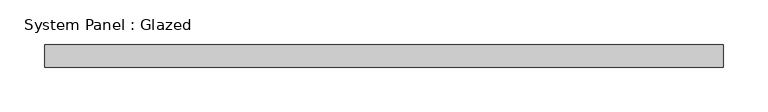
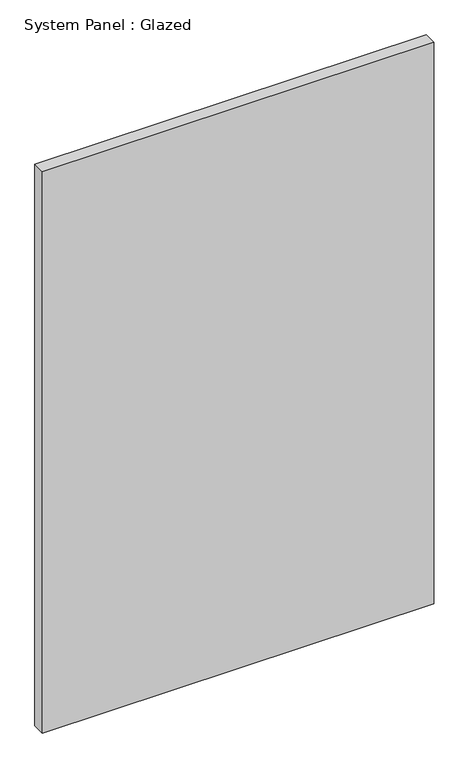
"""IFC4 building model written with IfcOpenShell, lengths in millimetres: plate geometry, System Panel : Glazed."""

from ifc_helpers import new_model, si_unit, origin, origin_with_axes, place, context, project, spatial, polyline, outline, extrude, source, transform, mapped, element, save


def system_panel_glazed_f269d4c8(model_context):
    return source(origin(), model_context, "Body", "SweptSolid", [
        extrude(outline(polyline([(381.0, 19.05), (-381.0, 19.05), (-381.0, 44.45), (381.0, 44.45), (381.0, 19.05)])), origin_with_axes(), (0.0, 0.0, 1.0), 1155.7),
    ])


if __name__ == "__main__":
    model = new_model("IFC4")
    model_context = context("Model", 3, world=origin())
    ifc_project = project(units=[si_unit("LENGTHUNIT", "METRE", prefix="MILLI")], contexts=[model_context])
    site = spatial("IfcSite", under=ifc_project)
    building = spatial("IfcBuilding", under=site)
    placement = place(None, origin())
    system_panel_glazed_shape = system_panel_glazed_f269d4c8(model_context)
    element("IfcPlate", 1, ObjectType="System Panel : Glazed", at=placement, inside=building, context=model_context, shape_type="MappedRepresentation", body=[
        mapped(system_panel_glazed_shape, transform((0.0, 0.0, 0.0), x_axis=(1.0, 0.0, 0.0), y_axis=(0.0, 1.0, 0.0), z_axis=(0.0, 0.0, 1.0))),
    ])
    save(model, "model.ifc")

# Revit data of these elements
# Type "System Panel : Glazed"
#   Construction Type Id = "GSP4R"
#   Analytic Construction = "1/8 in Pilkington single glazing"
#   Visual Light Transmittance = 0.9
#   Solar Heat Gain Coefficient = 0.86
#   Heat Transfer Coefficient (U) = 1.18115 BTU/(h·ft²·°F)
# Element 1 (IfcPlate, "System Panel : Glazed")
#   Materials on its faces: "Glass"
# Materials
#   "Glass": class "Glass", colour RGB 0 128 192, transparency 0.75, Description = "Soda Lime Glass", Cost = 0
